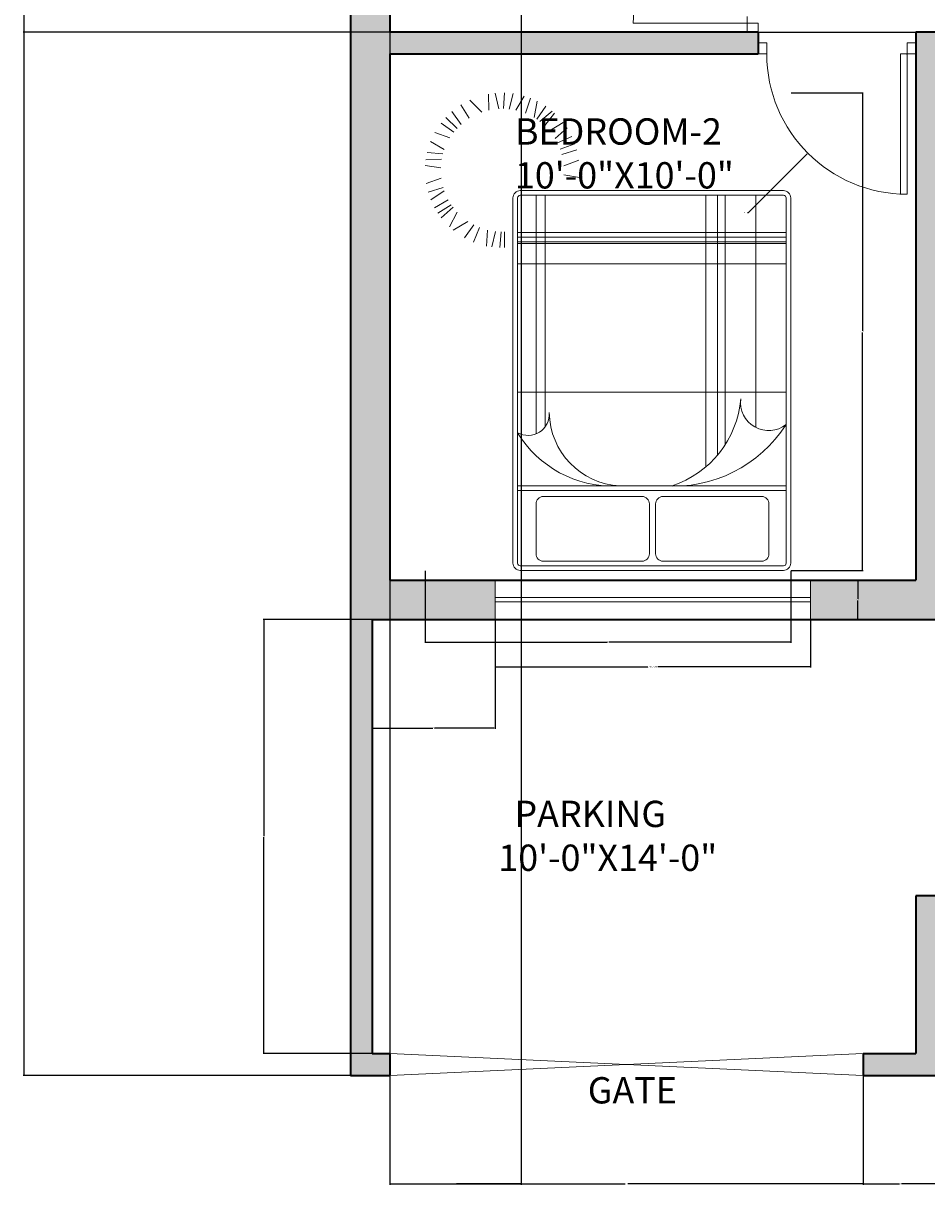
# Model space of a CAD drawing. Units: inches. Extents: x 126 to 477, y -70 to 465.
# Tile 1 of 5: x 126 to 332, y -70 to 195. Entities that reach past the tile are written whole.
import ezdxf

# ---------------------------------------------------------------- set-up
doc = ezdxf.new("R2010")
doc.units = ezdxf.units.IN
for name, color, linetype, lineweight in [('A-ANNO-DIMS', 2, 'Continuous', 18), ('A-ANNO-TEXT', 7, 'Continuous', 20), ('A-AREA-IDEN', 7, 'Continuous', 20), ('A-DOOR', 4, 'Continuous', 20), ('A-DOOR-GATE', 4, 'Continuous', 20), ('A-FURN', 8, 'Continuous', 18), ('A-GLAZ', 4, 'Continuous', 18), ('A-WALL', 7, 'Continuous', 35), ('A-WALL-PATT', 252, 'Continuous', 13)]:
    doc.layers.add(name, color=color, linetype=linetype, lineweight=lineweight)
doc.styles.get("Standard").update_dxf_attribs({"font": 'arial.ttf'})
doc.dimstyles.get("Standard").update_dxf_attribs({"dimtxt": 0.18, "dimasz": 0.18, "dimexe": 0.18, "dimexo": 0.0625, "dimgap": 0.09, "dimtad": 0, "dimtih": 1, "dimtoh": 1, "dimdec": 4, "dimzin": 0, "dimdsep": 46, "dimtxsty": 'Standard', "dimcen": 0.09, "dimadec": 0, "dimazin": 0, "dimtfac": 1, "dimtdec": 4, "dimtofl": 0, "dimtmove": 0, "dimatfit": 3, "dimfxl": 1, "dimtolj": 1, "dimtzin": 0, "dimarcsym": 0})

# ---------------------------------------------------------------- blocks, each defined once
blk = doc.blocks.new('A$C20A07B91')
for p, q in [((0.04, 2.5768), (1.46, 2.5768)), ((0, 0.5668), (0, 2.5368)), ((0.025, 0.5668), (0.025, 2.5368)), ((0.04, 2.5518), (1.46, 2.5518)), ((0.1577, 2.5267), (0.6896, 2.5267)), ((0.8032, 2.5267), (1.3351, 2.5267)), ((1.475, 2.5368), (1.475, 0.5668)), ((1.5, 2.5368), (1.5, 0.5668)), ((0.1177, 2.2177), (0.1177, 2.4867)), ((0.7296, 2.4867), (0.7296, 2.2177)), ((0.7632, 2.2177), (0.7632, 2.4867)), ((1.3751, 2.4867), (1.3751, 2.2177)), ((1.475, 2.1455), (0.025, 2.1455)), ((0.6896, 2.1777), (0.1577, 2.1777)), ((1.3351, 2.1777), (0.8032, 2.1777)), ((1.475, 2.1208), (0.025, 2.1208)), ((0.4594, 2.0186), (0.4594, 0.5518)), ((0.3952, 1.9538), (0.3952, 0.5518)), ((0.3537, 1.8973), (0.3537, 0.5518)), ((1.3735, 1.8387), (1.3735, 0.5518)), ((0.1881, 1.8055), (0.1881, 0.5518)), ((1.325, 1.7998), (1.325, 0.5518)), ((1.475, 1.6146), (0.025, 1.6146)), ((1.475, 0.9216), (0.025, 0.9216)), ((1.5448, 0.8348), (1.5455, 0.7499)), ((1.5699, 0.8347), (1.5633, 0.7501)), ((1.6143, 0.831), (1.5932, 0.7481)), ((1.6427, 0.8261), (1.6378, 0.7402)), ((1.475, 0.8127), (0.025, 0.8127)), ((1.475, 0.8028), (0.025, 0.8028)), ((1.475, 0.778), (0.025, 0.778)), ((1.475, 0.7533), (0.025, 0.7533)), ((1.7121, 0.8051), (1.6806, 0.7263)), ((1.7614, 0.7816), (1.7107, 0.7125)), ((1.8218, 0.7404), (1.7431, 0.6933)), ((1.8424, 0.7223), (1.8011, 0.6437)), ((1.8863, 0.6743), (1.8232, 0.6171)), ((1.9045, 0.6491), (1.833, 0.6034)), ((1.9224, 0.6197), (1.8494, 0.5764)), ((1.9429, 0.5771), (1.8708, 0.5282)), ((1.46, 0.5518), (0.04, 0.5518)), ((1.46, 0.5268), (0.04, 0.5268)), ((1.9576, 0.5356), (1.8768, 0.5097)), ((1.1413, 0.4558), (1.2253, 0.4415)), ((1.9686, 0.4882), (1.8872, 0.4594)), ((1.1432, 0.3625), (1.2252, 0.3937)), ((1.9739, 0.3913), (1.8896, 0.4048)), ((1.1543, 0.3074), (1.2354, 0.3323)), ((1.9636, 0.322), (1.8777, 0.3283)), ((1.9708, 0.3609), (1.8845, 0.3578)), ((1.2446, 0.3031), (1.1649, 0.2741)), ((1.1813, 0.2354), (1.2596, 0.2685)), ((1.9448, 0.2622), (1.8701, 0.3046)), ((1.2719, 0.2461), (1.2078, 0.1886)), ((1.3016, 0.2043), (1.2293, 0.1587)), ((1.8616, 0.1317), (1.8013, 0.1913)), ((1.888, 0.1627), (1.8187, 0.2117)), ((1.8402, 0.2426), (1.9212, 0.2128)), ((1.328, 0.1761), (1.2751, 0.1095)), ((1.2875, 0.0985), (1.3538, 0.154)), ((1.37, 0.1423), (1.3226, 0.0719)), ((1.3681, 0.0451), (1.3852, 0.1325)), ((1.7812, 0.065), (1.736, 0.1369)), ((1.7796, 0.17), (1.8287, 0.1002)), ((1.4315, 0.1093), (1.4056, 0.0283)), ((1.44, 0.0166), (1.4837, 0.0929)), ((1.5197, 0.0868), (1.499, 0.0039)), ((1.5447, 0), (1.5511, 0.0847)), ((1.5756, 0.0852), (1.5955, 0.0016)), ((1.6305, 0.0929), (1.6312, 0.0064)), ((1.6678, 0.1036), (1.7332, 0.0388))]:
    blk.add_line(p, q)
for centre, radius, start, end in [((0.04, 2.5368), 0.04, 90, 180), ((1.46, 2.5368), 0.04, 0, 90), ((0.04, 2.5368), 0.015, 90, 180), ((0.1577, 2.4867), 0.04, 90, 180), ((0.6896, 2.4867), 0.04, 0, 90), ((0.8032, 2.4867), 0.04, 90, 180), ((1.3351, 2.4867), 0.04, 0, 90), ((1.46, 2.5368), 0.015, 0, 90), ((0.1577, 2.2177), 0.04, 180, 270), ((0.6896, 2.2177), 0.04, 270, 0), ((0.8032, 2.2177), 0.04, 180, 270), ((1.3351, 2.2177), 0.04, 270, 0), ((0.6351, 1.3977), 0.7248, 86.01998, 147.31517), ((0.8125, 1.604), 0.5445, 108.37185, 175.10395), ((0.9022, 1.72), 0.4013, 0.68408, 87.06887), ((0.9629, 1.5212), 0.5999, 31.38578, 91.94583), ((0.1193, 1.6701), 0.1519, 352.59612, 128.40132), ((1.419, 1.7323), 0.1157, 61.08706, 183.75653), ((0.04, 0.5668), 0.04, 180, 270), ((0.04, 0.5668), 0.015, 180, 270), ((1.46, 0.5668), 0.04, 270, 0), ((1.46, 0.5668), 0.015, 270, 0)]:
    blk.add_arc(centre, radius, start, end)
blk = doc.blocks.new('DOOR-SINGLE-36IN')
for p, q in [((2, 34.5), (2, 2.5)), ((3.5, 34.46), (3.5, 2.5)), ((2, 2.5), (0, 2.5)), ((0, 0), (2, 0)), ((2, 0), (2, 2.5)), ((2, 2.5), (3.5, 2.5)), ((34, 0), (34, 2.5)), ((34, 2.5), (36, 2.5)), ((36, 0), (34, 0))]:
    blk.add_line(p, q)
blk.add_arc((2, 2.5), 32, 0, 90)
blk = doc.blocks.new('WIN-72IN')
for p, q in [((0, 0), (0, 9)), ((72, 0), (72, 9)), ((72, 5), (0, 5)), ((72, 4), (0, 4))]:
    blk.add_line(p, q)
blk = doc.blocks.new('*D11')
at = {"layer": 'A-ANNO-DIMS', "color": 0, "lineweight": -2, "transparency": 16777216}
for p, q in [((233.53, 58.82), (233.53, 47.9)), ((305.53, 58.82), (305.53, 47.9)), ((233.71, 48.08), (268.41, 48.08)), ((305.35, 48.08), (270.65, 48.08))]:
    blk.add_line(p, q, dxfattribs=at)
at = {"layer": 'A-ANNO-DIMS', "color": 0, "transparency": 16777216}
for points in [[(233.71, 48.11), (233.71, 48.05), (233.53, 48.08)], [(305.35, 48.11), (305.35, 48.05), (305.53, 48.08)]]:
    blk.add_solid(points, dxfattribs=at)
at = {"layer": 'Defpoints', "color": 0, "transparency": 16777216}
for p in [(233.53, 58.88), (305.53, 58.88), (305.53, 48.08)]:
    blk.add_point(p, dxfattribs=at)
at = {"layer": 'A-ANNO-DIMS', "color": 0, "transparency": 16777216, "insert": (269.53, 48.08), "char_height": 0.18, "attachment_point": 5}
blk.add_mtext('\\A1;WINDOW 72 TYP.', dxfattribs=at)
blk = doc.blocks.new('*D12')
at = {"layer": 'A-ANNO-DIMS', "color": 0, "lineweight": -2, "transparency": 16777216}
for p, q in [((305.6, 67.88), (316.51, 67.88)), ((316.33, 67.7), (316.33, 63.56)), ((316.33, 59.06), (316.33, 63.2)), ((305.6, 58.88), (316.51, 58.88))]:
    blk.add_line(p, q, dxfattribs=at)
at = {"layer": 'A-ANNO-DIMS', "color": 0, "transparency": 16777216}
for points in [[(316.3, 67.7), (316.36, 67.7), (316.33, 67.88)], [(316.3, 59.06), (316.36, 59.06), (316.33, 58.88)]]:
    blk.add_solid(points, dxfattribs=at)
at = {"layer": 'Defpoints', "color": 0, "transparency": 16777216}
for p in [(305.53, 67.88), (316.33, 67.88), (305.53, 58.88)]:
    blk.add_point(p, dxfattribs=at)
at = {"layer": 'A-ANNO-DIMS', "color": 0, "transparency": 16777216, "insert": (316.33, 63.38), "char_height": 0.18, "attachment_point": 5}
blk.add_mtext('\\A1;9 TYP.', dxfattribs=at)
blk = doc.blocks.new('*D17')
at = {"layer": 'A-ANNO-DIMS', "color": 0, "lineweight": -2, "transparency": 16777216}
for p, q in [((301.07, 178.98), (317.53, 178.98)), ((317.35, 178.8), (317.35, 124.71)), ((317.35, 70.24), (317.35, 124.34)), ((301.07, 70.06), (317.53, 70.06))]:
    blk.add_line(p, q, dxfattribs=at)
at = {"layer": 'A-ANNO-DIMS', "color": 0, "transparency": 16777216}
for points in [[(317.32, 178.8), (317.38, 178.8), (317.35, 178.98)], [(317.32, 70.24), (317.38, 70.24), (317.35, 70.06)]]:
    blk.add_solid(points, dxfattribs=at)
at = {"layer": 'Defpoints', "color": 0, "transparency": 16777216}
for p in [(301.01, 178.98), (301.01, 70.06), (317.35, 70.06)]:
    blk.add_point(p, dxfattribs=at)
at = {"layer": 'A-ANNO-DIMS', "color": 0, "transparency": 16777216, "insert": (317.35, 124.52), "char_height": 0.18, "attachment_point": 5}
blk.add_mtext('\\A1;BED GROUP 109', dxfattribs=at)
blk = doc.blocks.new('*D18')
at = {"layer": 'A-ANNO-DIMS', "color": 0, "lineweight": -2, "transparency": 16777216}
for p, q in [((217.58, 70), (217.58, 53.55)), ((301.01, 70), (301.01, 53.55)), ((217.76, 53.73), (259.08, 53.73)), ((300.83, 53.73), (259.51, 53.73))]:
    blk.add_line(p, q, dxfattribs=at)
at = {"layer": 'A-ANNO-DIMS', "color": 0, "transparency": 16777216}
for points in [[(217.76, 53.76), (217.76, 53.7), (217.58, 53.73)], [(300.83, 53.76), (300.83, 53.7), (301.01, 53.73)]]:
    blk.add_solid(points, dxfattribs=at)
at = {"layer": 'Defpoints', "color": 0, "transparency": 16777216}
for p in [(217.58, 70.06), (301.01, 70.06), (217.58, 53.73)]:
    blk.add_point(p, dxfattribs=at)
at = {"layer": 'A-ANNO-DIMS', "color": 0, "transparency": 16777216, "insert": (259.3, 53.73), "char_height": 0.18, "attachment_point": 5}
blk.add_mtext('\\A1;83', dxfattribs=at)
blk = doc.blocks.new('*D30')
at = {"layer": 'A-ANNO-DIMS', "color": 0, "lineweight": -2, "transparency": 16777216}
for p, q in [((200.47, 439.88), (125.92, 439.88)), ((126.1, 439.7), (126.1, 197.56)), ((126.1, -44.94), (126.1, 197.2)), ((200.47, -45.12), (125.92, -45.12))]:
    blk.add_line(p, q, dxfattribs=at)
at = {"layer": 'A-ANNO-DIMS', "color": 0, "transparency": 16777216}
for points in [[(126.07, 439.7), (126.13, 439.7), (126.1, 439.88)], [(126.07, -44.94), (126.13, -44.94), (126.1, -45.12)]]:
    blk.add_solid(points, dxfattribs=at)
at = {"layer": 'Defpoints', "color": 0, "transparency": 16777216}
for p in [(126.1, 439.88), (200.53, 439.88), (200.53, -45.12)]:
    blk.add_point(p, dxfattribs=at)
at = {"layer": 'A-ANNO-DIMS', "color": 0, "transparency": 16777216, "insert": (126.1, 197.38), "char_height": 0.18, "attachment_point": 5}
blk.add_mtext('\\A1;485', dxfattribs=at)
blk = doc.blocks.new('*D31')
at = {"layer": 'A-ANNO-DIMS', "color": 0, "lineweight": -2, "transparency": 16777216}
for p, q in [((209.53, 430.82), (209.53, -70.05)), ((239.53, 430.82), (239.53, -70.05)), ((209.71, -69.87), (224.31, -69.87)), ((239.35, -69.87), (224.75, -69.87))]:
    blk.add_line(p, q, dxfattribs=at)
at = {"layer": 'A-ANNO-DIMS', "color": 0, "transparency": 16777216}
for points in [[(209.71, -69.84), (209.71, -69.9), (209.53, -69.87)], [(239.35, -69.84), (239.35, -69.9), (239.53, -69.87)]]:
    blk.add_solid(points, dxfattribs=at)
at = {"layer": 'Defpoints', "color": 0, "transparency": 16777216}
for p in [(209.53, 430.88), (239.53, 430.88), (239.53, -69.87)]:
    blk.add_point(p, dxfattribs=at)
at = {"layer": 'A-ANNO-DIMS', "color": 0, "transparency": 16777216, "insert": (224.53, -69.87), "char_height": 0.18, "attachment_point": 5}
blk.add_mtext('\\A1;30', dxfattribs=at)
blk = doc.blocks.new('*D33')
at = {"layer": 'A-ANNO-DIMS', "color": 0, "lineweight": -2, "transparency": 16777216}
for p, q in [((205.47, 58.88), (180.6, 58.88)), ((180.78, 58.7), (180.78, 9.56)), ((180.78, -39.94), (180.78, 9.2)), ((205.47, -40.12), (180.6, -40.12))]:
    blk.add_line(p, q, dxfattribs=at)
at = {"layer": 'A-ANNO-DIMS', "color": 0, "transparency": 16777216}
for points in [[(180.75, 58.7), (180.81, 58.7), (180.78, 58.88)], [(180.75, -39.94), (180.81, -39.94), (180.78, -40.12)]]:
    blk.add_solid(points, dxfattribs=at)
at = {"layer": 'Defpoints', "color": 0, "transparency": 16777216}
for p in [(180.78, 58.88), (205.53, 58.88), (205.53, -40.12)]:
    blk.add_point(p, dxfattribs=at)
at = {"layer": 'A-ANNO-DIMS', "color": 0, "transparency": 16777216, "insert": (180.78, 9.38), "char_height": 0.18, "attachment_point": 5}
blk.add_mtext('\\A1;99', dxfattribs=at)
blk = doc.blocks.new('*D39')
at = {"layer": 'A-ANNO-DIMS', "color": 0, "lineweight": -2, "transparency": 16777216}
for p, q in [((209.53, -45.18), (209.53, -70.05)), ((317.53, -45.18), (317.53, -70.05)), ((209.71, -69.87), (263.25, -69.87)), ((317.35, -69.87), (263.81, -69.87))]:
    blk.add_line(p, q, dxfattribs=at)
at = {"layer": 'A-ANNO-DIMS', "color": 0, "transparency": 16777216}
for points in [[(209.71, -69.84), (209.71, -69.9), (209.53, -69.87)], [(317.35, -69.84), (317.35, -69.9), (317.53, -69.87)]]:
    blk.add_solid(points, dxfattribs=at)
at = {"layer": 'Defpoints', "color": 0, "transparency": 16777216}
for p in [(209.53, -45.12), (317.53, -45.12), (317.53, -69.87)]:
    blk.add_point(p, dxfattribs=at)
at = {"layer": 'A-ANNO-DIMS', "color": 0, "transparency": 16777216, "insert": (263.53, -69.87), "char_height": 0.18, "attachment_point": 5}
blk.add_mtext('\\A1;108', dxfattribs=at)
blk = doc.blocks.new('*D40')
at = {"layer": 'A-ANNO-DIMS', "color": 0, "lineweight": -2, "transparency": 16777216}
for p, q in [((317.53, -45.18), (317.53, -70.05)), ((334.53, -45.18), (334.53, -70.05)), ((317.71, -69.87), (325.82, -69.87)), ((334.35, -69.87), (326.24, -69.87))]:
    blk.add_line(p, q, dxfattribs=at)
at = {"layer": 'A-ANNO-DIMS', "color": 0, "transparency": 16777216}
for points in [[(317.71, -69.84), (317.71, -69.9), (317.53, -69.87)], [(334.35, -69.84), (334.35, -69.9), (334.53, -69.87)]]:
    blk.add_solid(points, dxfattribs=at)
at = {"layer": 'Defpoints', "color": 0, "transparency": 16777216}
for p in [(317.53, -45.12), (334.53, -45.12), (334.53, -69.87)]:
    blk.add_point(p, dxfattribs=at)
at = {"layer": 'A-ANNO-DIMS', "color": 0, "transparency": 16777216, "insert": (326.03, -69.87), "char_height": 0.18, "attachment_point": 5}
blk.add_mtext('\\A1;17', dxfattribs=at)
blk = doc.blocks.new('*D46')
at = {"layer": 'A-ANNO-DIMS', "color": 0, "lineweight": -2, "transparency": 16777216}
for p, q in [((205.53, 58.82), (205.53, 33.95)), ((233.53, 58.82), (233.53, 33.95)), ((205.71, 34.13), (219.31, 34.13)), ((233.35, 34.13), (219.75, 34.13))]:
    blk.add_line(p, q, dxfattribs=at)
at = {"layer": 'A-ANNO-DIMS', "color": 0, "transparency": 16777216}
for points in [[(205.71, 34.16), (205.71, 34.1), (205.53, 34.13)], [(233.35, 34.16), (233.35, 34.1), (233.53, 34.13)]]:
    blk.add_solid(points, dxfattribs=at)
at = {"layer": 'Defpoints', "color": 0, "transparency": 16777216}
for p in [(205.53, 58.88), (233.53, 58.88), (205.53, 34.13)]:
    blk.add_point(p, dxfattribs=at)
at = {"layer": 'A-ANNO-DIMS', "color": 0, "transparency": 16777216, "insert": (219.53, 34.13), "char_height": 0.18, "attachment_point": 5}
blk.add_mtext('\\A1;28', dxfattribs=at)
blk = doc.blocks.new('*D51')
at = {"layer": 'A-ANNO-DIMS', "color": 0, "lineweight": -2, "transparency": 16777216}
for p, q in [((293.6, 222.88), (476.46, 222.88)), ((476.28, 222.7), (476.28, 208.06)), ((476.28, 193.06), (476.28, 207.7)), ((293.6, 192.88), (476.46, 192.88))]:
    blk.add_line(p, q, dxfattribs=at)
at = {"layer": 'A-ANNO-DIMS', "color": 0, "transparency": 16777216}
for points in [[(476.25, 222.7), (476.31, 222.7), (476.28, 222.88)], [(476.25, 193.06), (476.31, 193.06), (476.28, 192.88)]]:
    blk.add_solid(points, dxfattribs=at)
at = {"layer": 'Defpoints', "color": 0, "transparency": 16777216}
for p in [(293.53, 222.88), (476.28, 222.88), (293.53, 192.88)]:
    blk.add_point(p, dxfattribs=at)
at = {"layer": 'A-ANNO-DIMS', "color": 0, "transparency": 16777216, "insert": (476.28, 207.88), "char_height": 0.18, "attachment_point": 5}
blk.add_mtext('\\A1;30', dxfattribs=at)
blk = doc.blocks.new('*D53')
at = {"layer": 'A-ANNO-DIMS', "color": 0, "lineweight": -2, "transparency": 16777216}
for p, q in [((200.47, 204.88), (125.92, 204.88)), ((126.1, 204.7), (126.1, 199.06)), ((126.1, 193.06), (126.1, 198.7)), ((209.47, 192.88), (125.92, 192.88))]:
    blk.add_line(p, q, dxfattribs=at)
at = {"layer": 'A-ANNO-DIMS', "color": 0, "transparency": 16777216}
for points in [[(126.07, 204.7), (126.13, 204.7), (126.1, 204.88)], [(126.07, 193.06), (126.13, 193.06), (126.1, 192.88)]]:
    blk.add_solid(points, dxfattribs=at)
at = {"layer": 'Defpoints', "color": 0, "transparency": 16777216}
for p in [(126.1, 204.88), (200.53, 204.88), (209.53, 192.88)]:
    blk.add_point(p, dxfattribs=at)
at = {"layer": 'A-ANNO-DIMS', "color": 0, "transparency": 16777216, "insert": (126.1, 198.88), "char_height": 0.18, "attachment_point": 5}
blk.add_mtext('\\A1;12', dxfattribs=at)
blk = doc.blocks.new('*D59')
at = {"layer": 'A-ANNO-DIMS', "color": 0, "lineweight": -2, "transparency": 16777216}
for p, q in [((327.44, 187.88), (327.62, 187.88)), ((327.53, 187.79), (327.53, 187.97)), ((291.33, 151.68), (304.78, 165.13)), ((291.15, 151.68), (291.33, 151.68))]:
    blk.add_line(p, q, dxfattribs=at)
at = {"layer": 'A-ANNO-DIMS', "color": 0, "transparency": 16777216}
blk.add_solid([(304.76, 165.15), (304.8, 165.1), (304.91, 165.25)], dxfattribs=at)
at = {"layer": 'Defpoints', "color": 0, "transparency": 16777216}
for p in [(327.53, 187.88), (304.91, 165.25)]:
    blk.add_point(p, dxfattribs=at)
at = {"layer": 'A-ANNO-DIMS', "color": 0, "transparency": 16777216, "insert": (290.65, 151.68), "char_height": 0.18, "attachment_point": 5}
blk.add_mtext('\\A1;3X R32', dxfattribs=at)

msp = doc.modelspace()

# ---------------------------------------------------------------- hatches: boundary and pattern name
at = {"layer": 'A-WALL-PATT'}
h = msp.add_hatch(color=256, dxfattribs=at)
h.dxf.hatch_style = 1
h.paths.add_polyline_path([(334.5333, -4.1194), (329.5333, -4.1194), (329.5333, -40.1194), (317.5333, -40.1194), (317.5333, -45.1194), (334.5333, -45.1194)])
h.paths.add_polyline_path([(205.5333, 58.8806), (233.5333, 58.8806), (233.5333, 67.8806), (209.5333, 67.8806), (209.5333, 187.8806), (293.5333, 187.8806), (293.5333, 192.8806), (209.5333, 192.8806), (209.5333, 204.8806), (200.5333, 204.8806), (200.5333, -45.1194), (209.5333, -45.1194), (209.5333, -40.1194), (205.5333, -40.1194)])
h = msp.add_hatch(color=256, dxfattribs=at)
h.dxf.hatch_style = 1
h.paths.add_polyline_path([(334.5333, 192.8806), (329.5333, 192.8806), (329.5333, 67.8806), (305.5333, 67.8806), (305.5333, 58.8806), (334.5333, 58.8806)])

# ---------------------------------------------------------------- linework, layer by layer
at = {"layer": 'A-DOOR'}
for p, q in [((291.0333, 194.8806), (291.0333, 196.3806)), ((265.0333, 194.8806), (291.0333, 194.8806)), ((291.0333, 192.8806), (291.0333, 194.8806)), ((291.0333, 194.8806), (293.5333, 194.8806)), ((291.0333, 194.8806), (291.0333, 194.8806)), ((293.5333, 194.8806), (293.5333, 192.8806))]:
    msp.add_line(p, q, dxfattribs=at)
msp.add_arc((291.0333, 194.8806), 26, 90, 180, dxfattribs=at)
at = {"layer": 'A-DOOR-GATE'}
for p, q in [((317.5333, -45.1194), (209.5333, -40.1194)), ((209.5333, -45.1194), (317.5333, -40.1194))]:
    msp.add_line(p, q, dxfattribs=at)
at = {"layer": 'A-WALL'}
for p, q in [((200.5333, 439.8806), (200.5333, -45.1194)), ((209.5333, 240.8806), (209.5333, 192.8806)), ((209.5333, 192.8806), (293.5333, 192.8806)), ((293.5333, 192.8806), (293.5333, 187.8806)), ((329.5333, 192.8806), (329.5333, 67.8806)), ((329.5333, 192.8806), (334.5333, 192.8806)), ((209.5333, 187.8806), (293.5333, 187.8806)), ((209.5333, 187.8806), (209.5333, 67.8806)), ((209.5333, 187.8806), (209.5333, 67.8806)), ((209.5333, 67.8806), (329.5333, 67.8806)), ((205.5333, 58.8806), (334.5333, 58.8806)), ((205.5333, 58.8806), (205.5333, -40.1194)), ((329.5333, -4.1194), (329.5333, -40.1194)), ((334.5333, -4.1194), (329.5333, -4.1194)), ((205.5333, -40.1194), (209.5333, -40.1194)), ((209.5333, -40.1194), (209.5333, -45.1194)), ((317.5333, -40.1194), (317.5333, -45.1194)), ((317.5333, -40.1194), (329.5333, -40.1194)), ((200.5333, -45.1194), (209.5333, -45.1194)), ((317.5333, -45.1194), (451.5333, -45.1194))]:
    msp.add_line(p, q, dxfattribs=at)

# ---------------------------------------------------------------- block references
at = {"layer": 'A-DOOR', "rotation": 180}
msp.add_blockref('DOOR-SINGLE-36IN', (329.5333, 190.3806), dxfattribs=at)
at = {"layer": 'A-FURN', "xscale": 42.26723658700153, "yscale": 42.26723658700153, "zscale": 42.26723658700153, "rotation": 180}
msp.add_blockref('A$C20A07B91', (301.0103, 178.9805), dxfattribs=at)
at = {"layer": 'A-GLAZ'}
msp.add_blockref('WIN-72IN', (233.5333, 58.8806), dxfattribs=at)

# ---------------------------------------------------------------- texts
at = {"layer": 'A-ANNO-TEXT', "insert": (254.6871, -45.5036), "char_height": 6, "attachment_point": 1}
msp.add_mtext_dynamic_manual_height_columns('GATE', width=47.476602, gutter_width=12.5, heights=[0], dxfattribs=at)
at = {"layer": 'A-AREA-IDEN', "char_height": 6, "attachment_point": 1}
for s, insert in [('BEDROOM-2\\P10\'-0"X10\'-0"', (238.0811, 173.1905)), ('  PARKING\\P10\'-0"X14\'-0"', (234.2862, 17.5415))]:
    msp.add_mtext_dynamic_manual_height_columns(s, width=53.344839, gutter_width=12.5, heights=[0], dxfattribs=dict(at, insert=insert))

# ---------------------------------------------------------------- dimensions: what is measured, and where the dimension line sits
at = {"layer": 'A-ANNO-DIMS'}
for base, p1, p2, angle, picture, middle in [((126.1001, 439.8806), (200.5333, -45.1194), (200.5333, 439.8806), 90, '*D30', (126.1001, 197.3806)), ((476.2833, 222.8806), (293.5333, 192.8806), (293.5333, 222.8806), 90, '*D51', (476.2833, 207.8806)), ((126.1001, 204.8806), (209.5333, 192.8806), (200.5333, 204.8806), 90, '*D53', (126.1001, 198.8806)), ((217.5805, 53.7276), (301.0103, 70.0649), (217.5805, 70.0649), 180, '*D18', (259.2954, 53.7276)), ((180.7833, 58.8806), (205.5333, -40.1194), (205.5333, 58.8806), 90, '*D33', (180.7833, 9.3806)), ((205.5333, 34.1306), (233.5333, 58.8806), (205.5333, 58.8806), 180, '*D46', (219.5333, 34.1306))]:
    dim = msp.add_linear_dim(base=base, p1=p1, p2=p2, angle=angle, dimstyle='Standard', override={"dimdec": 0, "dimlfac": 1, "dimrnd": 0, "dimzin": 0, "dimdsep": 46, "dimlunit": 2}, dxfattribs=at)
    dim.commit()
    dim.dimension.update_dxf_attribs({"geometry": picture, "text_midpoint": middle})
for base, p1, p2, picture, middle in [((239.5333, -69.8694), (209.5333, 430.8806), (239.5333, 430.8806), '*D31', (224.5333, -69.8694)), ((317.5333, -69.8694), (209.5333, -45.1194), (317.5333, -45.1194), '*D39', (263.5333, -69.8694)), ((334.5333, -69.8694), (317.5333, -45.1194), (334.5333, -45.1194), '*D40', (326.0333, -69.8694))]:
    dim = msp.add_linear_dim(base=base, p1=p1, p2=p2, dimstyle='Standard', override={"dimdec": 0, "dimlfac": 1, "dimrnd": 0, "dimzin": 0, "dimdsep": 46, "dimlunit": 2}, dxfattribs=at)
    dim.commit()
    dim.dimension.update_dxf_attribs({"geometry": picture, "text_midpoint": middle})
dim = msp.add_radius_dim(center=(327.5333, 187.8806), mpoint=(304.9061, 165.2531), text='3X <>', dimstyle='Standard', override={"dimdec": 0, "dimlfac": 1, "dimrnd": 0, "dimzin": 0, "dimdsep": 46, "dimlunit": 2}, dxfattribs=at)
dim.commit()
dim.dimension.update_dxf_attribs({"geometry": '*D59', "text_midpoint": (290.6523, 151.6765), "dimtype": 164})
for base, p1, p2, angle, text, picture, middle in [((317.3476, 70.0649), (301.0103, 178.9805), (301.0103, 70.0649), 270, 'BED GROUP <>', '*D17', (317.3476, 124.5227)), ((316.3333, 67.8806), (305.5333, 58.8806), (305.5333, 67.8806), 90, '<> TYP.', '*D12', (316.3333, 63.3806))]:
    dim = msp.add_linear_dim(base=base, p1=p1, p2=p2, angle=angle, text=text, dimstyle='Standard', override={"dimdec": 0, "dimlfac": 1, "dimrnd": 0, "dimzin": 0, "dimdsep": 46, "dimlunit": 2}, dxfattribs=at)
    dim.commit()
    dim.dimension.update_dxf_attribs({"geometry": picture, "text_midpoint": middle})
dim = msp.add_linear_dim(base=(305.5333, 48.0806), p1=(233.5333, 58.8806), p2=(305.5333, 58.8806), text='WINDOW <> TYP.', dimstyle='Standard', override={"dimdec": 0, "dimlfac": 1, "dimrnd": 0, "dimzin": 0, "dimdsep": 46, "dimlunit": 2}, dxfattribs=at)
dim.commit()
dim.dimension.update_dxf_attribs({"geometry": '*D11', "text_midpoint": (269.5333, 48.0806)})

doc.saveas('drawing.dxf')
